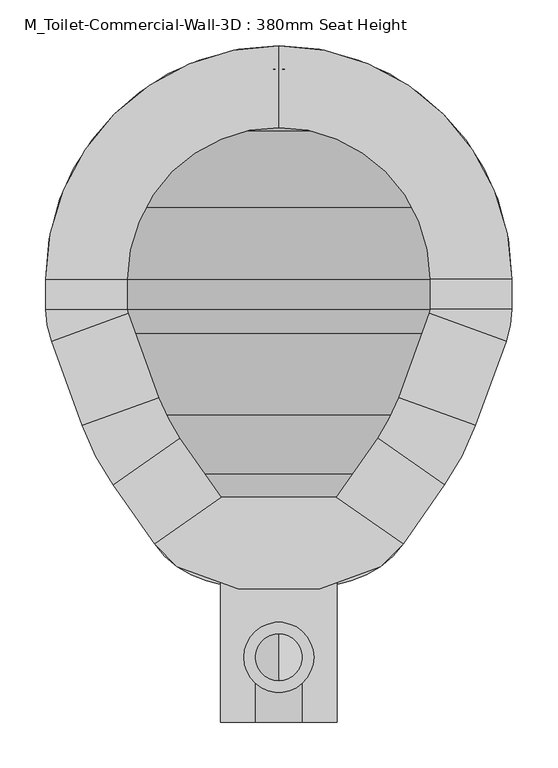
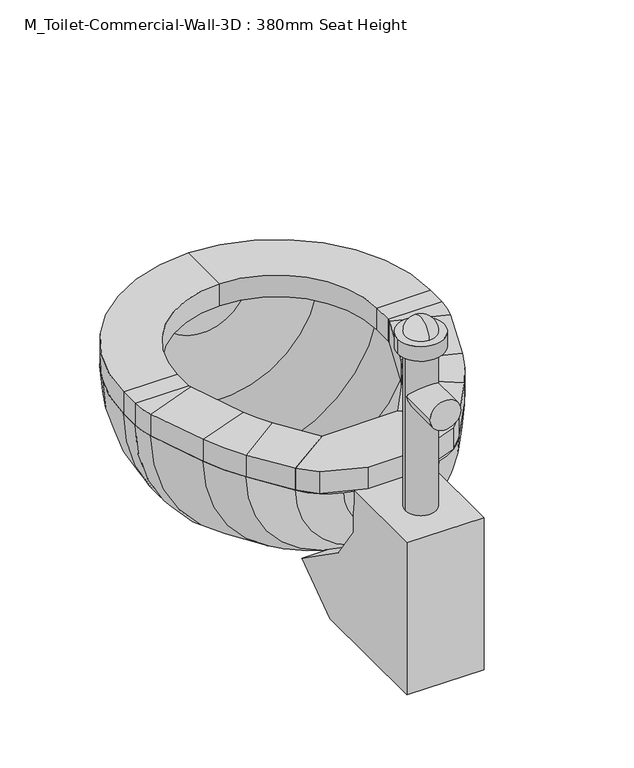
"""IFC4 building model written with IfcOpenShell, lengths in millimetres: flow terminal geometry, M_Toilet-Commercial-Wall-3D : 380mm Seat Height."""

from ifc_helpers import new_model, si_unit, point, frame, frame_2d, origin, place, context, project, spatial, polyline, circle_curve, ellipse_curve, trimmed, segment, composite_curve, outline, extrude, source, transform, mapped, element, save
from ifc_brep_helpers import plane_surface, cylinder_surface, revolved_surface, advanced_brep


def m_toilet_commercial_wall_3d_380mm_seat_height_4e8788ad(model_context):
    return source(origin(), model_context, "Body", "SolidModel", [
        extrude(outline(polyline([(302.8037941, 341.9), (302.8037941, 268.296452), (346.5103185, 205.8770663), (450.5426282, 133.0328588), (370.0454017, 76.2), (150.0, 76.2), (150.0, 341.9), (302.8037941, 341.9)])), frame((341.4031538, 0.0, 0.0), z_axis=(1.0, 0.0, 0.0), x_axis=(0.0, 1.0, 0.0)), (0.0, 0.0, 1.0), 127.0),
        extrude(outline(composite_curve([segment(trimmed(circle_curve(frame_2d((404.9031538, 220.5352737)), 25.4), [point((379.5031538, 220.5352737))], [point((430.3031538, 220.5352737))], False, "CARTESIAN"), True, "CONTINUOUS"), segment(trimmed(circle_curve(frame_2d((404.9031538, 220.5352737)), 25.4), [point((430.3031538, 220.5352737))], [point((379.5031538, 220.5352737))], False, "CARTESIAN"), True, "CONTINUOUS")], self_intersect=False)), frame((0.0, 0.0, 341.9), z_axis=(0.0, 0.0, 1.0), x_axis=(1.0, 0.0, 0.0)), (0.0, 0.0, 1.0), 279.4),
        extrude(outline(composite_curve([segment(trimmed(circle_curve(frame_2d((543.2113641, 404.9031538)), 25.4), [point((543.2113641, 379.5031538))], [point((543.2113641, 430.3031538))], False, "CARTESIAN"), True, "CONTINUOUS"), segment(trimmed(circle_curve(frame_2d((543.2113641, 404.9031538)), 25.4), [point((543.2113641, 430.3031538))], [point((543.2113641, 379.5031538))], False, "CARTESIAN"), True, "CONTINUOUS")], self_intersect=False)), frame((0.0, 150.0, 0.0), z_axis=(0.0, 1.0, 0.0), x_axis=(0.0, 0.0, 1.0)), (0.0, 0.0, 1.0), 70.64375),
        extrude(outline(composite_curve([segment(trimmed(circle_curve(frame_2d((404.9031538, 220.5352737)), 38.1), [point((366.8031538, 220.5352737))], [point((443.0031538, 220.5352737))], False, "CARTESIAN"), True, "CONTINUOUS"), segment(trimmed(circle_curve(frame_2d((404.9031538, 220.5352737)), 38.1), [point((443.0031538, 220.5352737))], [point((366.8031538, 220.5352737))], False, "CARTESIAN"), True, "CONTINUOUS")], self_intersect=False)), frame((0.0, 0.0, 621.3), z_axis=(0.0, 0.0, 1.0), x_axis=(1.0, 0.0, 0.0)), (0.0, 0.0, 1.0), 25.4),
        advanced_brep(
        [(404.9031538, 194.9176912, 646.7), (404.9031538, 246.1528563, 646.7), (404.9031538, 220.5352737, 672.3175826), (404.9031538, 220.5352737, 646.7)],
        [
            (0, 1, circle_curve(frame((404.9031538, 220.5352737, 646.7), z_axis=(0.0, 0.0, 1.0), x_axis=(0.0, 1.0, 0.0)), 25.6175826)),
            (1, 2, circle_curve(frame((404.9031538, 220.5352737, 646.7), z_axis=(1.0, 0.0, 0.0), x_axis=(0.0, -1.0, 0.0)), 25.6175826)),
            (2, 0, circle_curve(frame((404.9031538, 220.5352737, 646.7), z_axis=(1.0, 0.0, 0.0), x_axis=(0.0, 1.0, 0.0)), 25.6175826)),
            (1, 0, circle_curve(frame((404.9031538, 220.5352737, 646.7), z_axis=(0.0, 0.0, 1.0), x_axis=(0.0, 1.0, 0.0)), 25.6175826)),
            (3, 1),
            (0, 3),
        ],
        [
            revolved_surface(trimmed(ellipse_curve(frame((404.9031538, 220.5352737, 646.7), z_axis=(-1.0, 0.0, 0.0), x_axis=(0.0, -1.0, 0.0)), 25.6175826, 25.6175826), [point((404.9031538, 220.5352737, 672.3175826))], [point((404.9031538, 246.1528563, 646.7))], True, "CARTESIAN"), (404.9031538, 220.5352737, 711.3277273), (0.0, 0.0, -1.0)),
            plane_surface(frame((404.9031538, 220.5352737, 646.7), z_axis=(0.0, 0.0, -1.0), x_axis=(0.0, 1.0, 0.0))),
        ],
        [
            (0, [[1, 2, 3]]),
            (0, [[4, -3, -2]]),
            (1, [[5, -1, 6]]),
            (1, [[-6, -4, -5]]),
        ],
    ),
        advanced_brep(
        [(491.7762702, 871.2819257, 341.9), (404.9031538, 886.6, 341.9), (404.9031538, 861.2, 341.9), (483.0889586, 847.4137331, 341.9), (566.547764, 794.2446102, 341.9), (619.7168869, 710.7858048, 341.9), (633.5031538, 632.6, 341.9), (633.5031538, 599.7148212, 341.9), (628.9077315, 573.6528863, 341.9), (596.6355667, 484.9858422, 341.9), (562.9565296, 420.2890139, 341.9), (525.0728964, 366.1855786, 341.9), (468.1430637, 326.3228806, 341.9), (404.9031538, 309.3777978, 341.9), (404.9031538, 283.0817829, 341.9), (483.6469009, 304.1811063, 341.9), (540.5767337, 344.0438043, 341.9), (585.6810159, 408.4593951, 341.9), (619.360053, 473.1562234, 341.9), (652.7759241, 564.9655747, 341.9), (658.9031538, 599.7148212, 341.9), (658.9031538, 632.6, 341.9), (643.5850795, 719.4731164, 341.9), (584.5082762, 812.2051224, 341.9), (318.0300374, 871.2819257, 341.9), (225.2980314, 812.2051224, 341.9), (166.2212281, 719.4731164, 341.9), (150.9031538, 632.6, 341.9), (150.9031538, 599.7148212, 341.9), (157.0303835, 564.9655747, 341.9), (190.4462546, 473.1562234, 341.9), (224.1252917, 408.4593951, 341.9), (269.229574, 344.0438043, 341.9), (326.1594067, 304.1811063, 341.9), (341.663244, 326.3228806, 341.9), (284.7334112, 366.1855786, 341.9), (246.849778, 420.2890139, 341.9), (213.1707409, 484.9858422, 341.9), (180.8985761, 573.6528863, 341.9), (176.3031538, 599.7148212, 341.9), (176.3031538, 632.6, 341.9), (190.0894207, 710.7858048, 341.9), (243.2585436, 794.2446102, 341.9), (326.7173491, 847.4137331, 341.9)],
        [
            (0, 1, circle_curve(frame((404.9031538, 632.6, 341.9), z_axis=(0.0, 0.0, 1.0), x_axis=(1.0, 0.0, 0.0)), 254.0)),
            (1, 2),
            (2, 3, circle_curve(frame((404.9031538, 632.6, 341.9), z_axis=(0.0, 0.0, -1.0), x_axis=(1.0, 0.0, 0.0)), 228.6)),
            (3, 4, circle_curve(frame((404.9031538, 632.6, 341.9), z_axis=(0.0, 0.0, -1.0), x_axis=(1.0, 0.0, 0.0)), 228.6)),
            (4, 5, circle_curve(frame((404.9031538, 632.6, 341.9), z_axis=(0.0, 0.0, -1.0), x_axis=(1.0, 0.0, 0.0)), 228.6)),
            (5, 6, circle_curve(frame((404.9031538, 632.6, 341.9), z_axis=(0.0, 0.0, -1.0), x_axis=(1.0, 0.0, 0.0)), 228.6)),
            (6, 7),
            (7, 8, circle_curve(frame((557.3031538, 599.7148212, 341.9), z_axis=(0.0, 0.0, -1.0), x_axis=(1.0, 0.0, 0.0)), 76.2)),
            (8, 9),
            (9, 10, circle_curve(frame((334.0854485, 580.5462703, 341.9), z_axis=(0.0, 0.0, -1.0), x_axis=(1.0, 0.0, 0.0)), 279.4)),
            (10, 11),
            (11, 12, circle_curve(frame((441.8470487, 424.4609446, 341.9), z_axis=(0.0, 0.0, -1.0), x_axis=(1.0, 0.0, 0.0)), 101.6)),
            (12, 13),
            (13, 14),
            (14, 15),
            (15, 16, circle_curve(frame((457.350886, 402.3191703, 341.9), z_axis=(0.0, 0.0, 1.0), x_axis=(1.0, 0.0, 0.0)), 101.6)),
            (16, 17),
            (17, 18, circle_curve(frame((356.8099347, 568.7166514, 341.9), z_axis=(0.0, 0.0, 1.0), x_axis=(1.0, 0.0, 0.0)), 279.4)),
            (18, 19),
            (19, 20, circle_curve(frame((557.3031538, 599.7148212, 341.9), z_axis=(0.0, 0.0, 1.0), x_axis=(1.0, 0.0, 0.0)), 101.6)),
            (20, 21),
            (21, 22, circle_curve(frame((404.9031538, 632.6, 341.9), z_axis=(0.0, 0.0, 1.0), x_axis=(1.0, 0.0, 0.0)), 254.0)),
            (22, 23, circle_curve(frame((404.9031538, 632.6, 341.9), z_axis=(0.0, 0.0, 1.0), x_axis=(1.0, 0.0, 0.0)), 254.0)),
            (23, 0, circle_curve(frame((404.9031538, 632.6, 341.9), z_axis=(0.0, 0.0, 1.0), x_axis=(1.0, 0.0, 0.0)), 254.0)),
            (24, 25, circle_curve(frame((404.9031538, 632.6, 341.9), z_axis=(0.0, 0.0, 1.0), x_axis=(-1.0, 0.0, 0.0)), 254.0)),
            (25, 26, circle_curve(frame((404.9031538, 632.6, 341.9), z_axis=(0.0, 0.0, 1.0), x_axis=(-1.0, 0.0, 0.0)), 254.0)),
            (26, 27, circle_curve(frame((404.9031538, 632.6, 341.9), z_axis=(0.0, 0.0, 1.0), x_axis=(-1.0, 0.0, 0.0)), 254.0)),
            (27, 28),
            (28, 29, circle_curve(frame((252.5031538, 599.7148212, 341.9), z_axis=(0.0, 0.0, 1.0), x_axis=(-1.0, 0.0, 0.0)), 101.6)),
            (29, 30),
            (30, 31, circle_curve(frame((452.9963729, 568.7166514, 341.9), z_axis=(0.0, 0.0, 1.0), x_axis=(-1.0, 0.0, 0.0)), 279.4)),
            (31, 32),
            (32, 33, circle_curve(frame((352.4554217, 402.3191703, 341.9), z_axis=(0.0, 0.0, 1.0), x_axis=(-1.0, 0.0, 0.0)), 101.6)),
            (33, 14),
            (13, 34),
            (34, 35, circle_curve(frame((367.9592589, 424.4609446, 341.9), z_axis=(0.0, 0.0, -1.0), x_axis=(-1.0, 0.0, 0.0)), 101.6)),
            (35, 36),
            (36, 37, circle_curve(frame((475.7208592, 580.5462703, 341.9), z_axis=(0.0, 0.0, -1.0), x_axis=(-1.0, 0.0, 0.0)), 279.4)),
            (37, 38),
            (38, 39, circle_curve(frame((252.5031538, 599.7148212, 341.9), z_axis=(0.0, 0.0, -1.0), x_axis=(-1.0, 0.0, 0.0)), 76.2)),
            (39, 40),
            (40, 41, circle_curve(frame((404.9031538, 632.6, 341.9), z_axis=(0.0, 0.0, -1.0), x_axis=(-1.0, 0.0, 0.0)), 228.6)),
            (41, 42, circle_curve(frame((404.9031538, 632.6, 341.9), z_axis=(0.0, 0.0, -1.0), x_axis=(-1.0, 0.0, 0.0)), 228.6)),
            (42, 43, circle_curve(frame((404.9031538, 632.6, 341.9), z_axis=(0.0, 0.0, -1.0), x_axis=(-1.0, 0.0, 0.0)), 228.6)),
            (43, 2, circle_curve(frame((404.9031538, 632.6, 341.9), z_axis=(0.0, 0.0, -1.0), x_axis=(-1.0, 0.0, 0.0)), 228.6)),
            (1, 24, circle_curve(frame((404.9031538, 632.6, 341.9), z_axis=(0.0, 0.0, 1.0), x_axis=(-1.0, 0.0, 0.0)), 254.0)),
            (0, 24, circle_curve(frame((404.9031538, 871.2819257, 341.9), z_axis=(0.0, 1.0, 0.0), x_axis=(1.0, 0.0, 0.0)), 86.8731164)),
            (43, 3, circle_curve(frame((404.9031538, 847.4137331, 341.9), z_axis=(0.0, -1.0, 0.0), x_axis=(1.0, 0.0, 0.0)), 78.1858048)),
            (42, 4, circle_curve(frame((404.9031538, 794.2446102, 341.9), z_axis=(0.0, -1.0, 0.0), x_axis=(1.0, 0.0, 0.0)), 161.6446102)),
            (41, 5, circle_curve(frame((404.9031538, 710.7858048, 341.9), z_axis=(0.0, -1.0, 0.0), x_axis=(1.0, 0.0, 0.0)), 214.8137331)),
            (40, 6, circle_curve(frame((404.9031538, 632.6, 341.9), z_axis=(0.0, -1.0, 0.0), x_axis=(1.0, 0.0, 0.0)), 228.6)),
            (39, 7, circle_curve(frame((404.9031538, 599.7148212, 341.9), z_axis=(0.0, -1.0, 0.0), x_axis=(1.0, 0.0, 0.0)), 228.6)),
            (38, 8, circle_curve(frame((404.9031538, 573.6528863, 341.9), z_axis=(0.0, -1.0, 0.0), x_axis=(1.0, 0.0, 0.0)), 224.0045777)),
            (37, 9, circle_curve(frame((404.9031538, 484.9858422, 341.9), z_axis=(0.0, -1.0, 0.0), x_axis=(1.0, 0.0, 0.0)), 191.7324129)),
            (36, 10, circle_curve(frame((404.9031538, 420.2890139, 341.9), z_axis=(0.0, -1.0, 0.0), x_axis=(1.0, 0.0, 0.0)), 158.0533758)),
            (35, 11, circle_curve(frame((404.9031538, 366.1855786, 341.9), z_axis=(0.0, -1.0, 0.0), x_axis=(1.0, 0.0, 0.0)), 120.1697426)),
            (34, 12, circle_curve(frame((404.9031538, 326.3228806, 341.9), z_axis=(0.0, -1.0, 0.0), x_axis=(1.0, 0.0, 0.0)), 63.2399099)),
            (33, 15, circle_curve(frame((404.9031538, 304.1811063, 341.9), z_axis=(0.0, -1.0, 0.0), x_axis=(1.0, 0.0, 0.0)), 78.7437471)),
            (32, 16, circle_curve(frame((404.9031538, 344.0438043, 341.9), z_axis=(0.0, -1.0, 0.0), x_axis=(1.0, 0.0, 0.0)), 135.6735798)),
            (31, 17, circle_curve(frame((404.9031538, 408.4593951, 341.9), z_axis=(0.0, -1.0, 0.0), x_axis=(1.0, 0.0, 0.0)), 180.7778621)),
            (30, 18, circle_curve(frame((404.9031538, 473.1562234, 341.9), z_axis=(0.0, -1.0, 0.0), x_axis=(1.0, 0.0, 0.0)), 214.4568992)),
            (29, 19, circle_curve(frame((404.9031538, 564.9655747, 341.9), z_axis=(0.0, -1.0, 0.0), x_axis=(1.0, 0.0, 0.0)), 247.8727703)),
            (28, 20, circle_curve(frame((404.9031538, 599.7148212, 341.9), z_axis=(0.0, -1.0, 0.0), x_axis=(1.0, 0.0, 0.0)), 254.0)),
            (27, 21, circle_curve(frame((404.9031538, 632.6, 341.9), z_axis=(0.0, -1.0, 0.0), x_axis=(1.0, 0.0, 0.0)), 254.0)),
            (26, 22, circle_curve(frame((404.9031538, 719.4731164, 341.9), z_axis=(0.0, -1.0, 0.0), x_axis=(1.0, 0.0, 0.0)), 238.6819257)),
            (25, 23, circle_curve(frame((404.9031538, 812.2051224, 341.9), z_axis=(0.0, -1.0, 0.0), x_axis=(1.0, 0.0, 0.0)), 179.6051224)),
        ],
        [
            plane_surface(frame((404.9031538, 991.8102448, 341.9), z_axis=(0.0, 0.0, 1.0), x_axis=(1.0, 0.0, 0.0))),
            plane_surface(frame((404.9031538, 991.8102448, 341.9), z_axis=(0.0, 0.0, 1.0), x_axis=(-1.0, 0.0, 0.0))),
            revolved_surface(trimmed(ellipse_curve(frame((404.9031538, 632.6, 341.9), z_axis=(0.0, 0.0, 1.0), x_axis=(1.0, 0.0, 0.0)), 254.0, 254.0), [point((491.7762702, 871.2819257, 341.9))], [point((404.9031538, 886.6, 341.9))], True, "CARTESIAN"), (404.9031538, 991.8102448, 341.9), (0.0, 1.0, 0.0)),
            revolved_surface(trimmed(ellipse_curve(frame((404.9031538, 632.6, 341.9), z_axis=(0.0, 0.0, -1.0), x_axis=(1.0, 0.0, 0.0)), 228.6, 228.6), [point((404.9031538, 861.2, 341.9))], [point((483.0889586, 847.4137331, 341.9))], True, "CARTESIAN"), (404.9031538, 991.8102448, 341.9), (0.0, 1.0, 0.0)),
            revolved_surface(trimmed(ellipse_curve(frame((404.9031538, 632.6, 341.9), z_axis=(0.0, 0.0, -1.0), x_axis=(1.0, 0.0, 0.0)), 228.6, 228.6), [point((483.0889586, 847.4137331, 341.9))], [point((566.547764, 794.2446102, 341.9))], True, "CARTESIAN"), (404.9031538, 991.8102448, 341.9), (0.0, 1.0, 0.0)),
            revolved_surface(trimmed(ellipse_curve(frame((404.9031538, 632.6, 341.9), z_axis=(0.0, 0.0, -1.0), x_axis=(1.0, 0.0, 0.0)), 228.6, 228.6), [point((566.547764, 794.2446102, 341.9))], [point((619.7168869, 710.7858048, 341.9))], True, "CARTESIAN"), (404.9031538, 991.8102448, 341.9), (0.0, 1.0, 0.0)),
            revolved_surface(trimmed(ellipse_curve(frame((404.9031538, 632.6, 341.9), z_axis=(0.0, 0.0, -1.0), x_axis=(1.0, 0.0, 0.0)), 228.6, 228.6), [point((619.7168869, 710.7858048, 341.9))], [point((633.5031538, 632.6, 341.9))], True, "CARTESIAN"), (404.9031538, 991.8102448, 341.9), (0.0, 1.0, 0.0)),
            revolved_surface(polyline([(633.5031538, 632.6, 341.9), (633.5031538, 599.7148212, 341.9)]), (404.9031538, 991.8102448, 341.9), (0.0, 1.0, 0.0)),
            revolved_surface(trimmed(ellipse_curve(frame((557.3031538, 599.7148212, 341.9), z_axis=(0.0, 0.0, -1.0), x_axis=(1.0, 0.0, 0.0)), 76.2, 76.2), [point((633.5031538, 599.7148212, 341.9))], [point((628.9077315, 573.6528863, 341.9))], True, "CARTESIAN"), (404.9031538, 991.8102448, 341.9), (0.0, 1.0, 0.0)),
            revolved_surface(polyline([(628.9077315, 573.6528863, 341.9), (596.6355667, 484.9858422, 341.9)]), (404.9031538, 991.8102448, 341.9), (0.0, 1.0, 0.0)),
            revolved_surface(trimmed(ellipse_curve(frame((334.0854485, 580.5462703, 341.9), z_axis=(0.0, 0.0, -1.0), x_axis=(1.0, 0.0, 0.0)), 279.4, 279.4), [point((596.6355667, 484.9858422, 341.9))], [point((562.9565296, 420.2890139, 341.9))], True, "CARTESIAN"), (404.9031538, 991.8102448, 341.9), (0.0, 1.0, 0.0)),
            revolved_surface(polyline([(562.9565296, 420.2890139, 341.9), (525.0728964, 366.1855786, 341.9)]), (404.9031538, 991.8102448, 341.9), (0.0, 1.0, 0.0)),
            revolved_surface(trimmed(ellipse_curve(frame((441.8470487, 424.4609446, 341.9), z_axis=(0.0, 0.0, -1.0), x_axis=(1.0, 0.0, 0.0)), 101.6, 101.6), [point((525.0728964, 366.1855786, 341.9))], [point((468.1430637, 326.3228806, 341.9))], True, "CARTESIAN"), (404.9031538, 991.8102448, 341.9), (0.0, 1.0, 0.0)),
            revolved_surface(polyline([(468.1430637, 326.3228806, 341.9), (404.9031538, 309.3777978, 341.9)]), (404.9031538, 991.8102448, 341.9), (0.0, 1.0, 0.0)),
            revolved_surface(polyline([(404.9031538, 283.0817829, 341.9), (483.6469009, 304.1811063, 341.9)]), (404.9031538, 991.8102448, 341.9), (0.0, 1.0, 0.0)),
            revolved_surface(trimmed(ellipse_curve(frame((457.350886, 402.3191703, 341.9), z_axis=(0.0, 0.0, 1.0), x_axis=(1.0, 0.0, 0.0)), 101.6, 101.6), [point((483.6469009, 304.1811063, 341.9))], [point((540.5767337, 344.0438043, 341.9))], True, "CARTESIAN"), (404.9031538, 991.8102448, 341.9), (0.0, 1.0, 0.0)),
            revolved_surface(polyline([(540.5767337, 344.0438043, 341.9), (585.6810159, 408.4593951, 341.9)]), (404.9031538, 991.8102448, 341.9), (0.0, 1.0, 0.0)),
            revolved_surface(trimmed(ellipse_curve(frame((356.8099347, 568.7166514, 341.9), z_axis=(0.0, 0.0, 1.0), x_axis=(1.0, 0.0, 0.0)), 279.4, 279.4), [point((585.6810159, 408.4593951, 341.9))], [point((619.360053, 473.1562234, 341.9))], True, "CARTESIAN"), (404.9031538, 991.8102448, 341.9), (0.0, 1.0, 0.0)),
            revolved_surface(polyline([(619.360053, 473.1562234, 341.9), (652.7759241, 564.9655747, 341.9)]), (404.9031538, 991.8102448, 341.9), (0.0, 1.0, 0.0)),
            revolved_surface(trimmed(ellipse_curve(frame((557.3031538, 599.7148212, 341.9), z_axis=(0.0, 0.0, 1.0), x_axis=(1.0, 0.0, 0.0)), 101.6, 101.6), [point((652.7759241, 564.9655747, 341.9))], [point((658.9031538, 599.7148212, 341.9))], True, "CARTESIAN"), (404.9031538, 991.8102448, 341.9), (0.0, 1.0, 0.0)),
            cylinder_surface(frame((404.9031538, 991.8102448, 341.9), z_axis=(0.0, 1.0, 0.0), x_axis=(1.0, 0.0, 0.0)), 254.0),
            revolved_surface(trimmed(ellipse_curve(frame((404.9031538, 632.6, 341.9), z_axis=(0.0, 0.0, 1.0), x_axis=(1.0, 0.0, 0.0)), 254.0, 254.0), [point((658.9031538, 632.6, 341.9))], [point((643.5850795, 719.4731164, 341.9))], True, "CARTESIAN"), (404.9031538, 991.8102448, 341.9), (0.0, 1.0, 0.0)),
            revolved_surface(trimmed(ellipse_curve(frame((404.9031538, 632.6, 341.9), z_axis=(0.0, 0.0, 1.0), x_axis=(1.0, 0.0, 0.0)), 254.0, 254.0), [point((643.5850795, 719.4731164, 341.9))], [point((584.5082762, 812.2051224, 341.9))], True, "CARTESIAN"), (404.9031538, 991.8102448, 341.9), (0.0, 1.0, 0.0)),
            revolved_surface(trimmed(ellipse_curve(frame((404.9031538, 632.6, 341.9), z_axis=(0.0, 0.0, 1.0), x_axis=(1.0, 0.0, 0.0)), 254.0, 254.0), [point((584.5082762, 812.2051224, 341.9))], [point((491.7762702, 871.2819257, 341.9))], True, "CARTESIAN"), (404.9031538, 991.8102448, 341.9), (0.0, 1.0, 0.0)),
        ],
        [
            (0, [[1, 2, 3, 4, 5, 6, 7, 8, 9, 10, 11, 12, 13, 14, 15, 16, 17, 18, 19, 20, 21, 22, 23, 24]]),
            (1, [[25, 26, 27, 28, 29, 30, 31, 32, 33, 34, -14, 35, 36, 37, 38, 39, 40, 41, 42, 43, 44, 45, -2, 46]]),
            (2, [[-1, 47, -46]]),
            (3, [[48, -3, -45]]),
            (4, [[49, -4, -48, -44]]),
            (5, [[50, -5, -49, -43]]),
            (6, [[51, -6, -50, -42]]),
            (7, [[52, -7, -51, -41]]),
            (8, [[53, -8, -52, -40]]),
            (9, [[54, -9, -53, -39]]),
            (10, [[55, -10, -54, -38]]),
            (11, [[56, -11, -55, -37]]),
            (12, [[57, -12, -56, -36]]),
            (13, [[-13, -57, -35]]),
            (14, [[58, -15, -34]]),
            (15, [[59, -16, -58, -33]]),
            (16, [[60, -17, -59, -32]]),
            (17, [[61, -18, -60, -31]]),
            (18, [[62, -19, -61, -30]]),
            (19, [[63, -20, -62, -29]]),
            (20, [[64, -21, -63, -28]]),
            (21, [[65, -22, -64, -27]]),
            (22, [[66, -23, -65, -26]]),
            (23, [[-47, -24, -66, -25]]),
        ],
    ),
        advanced_brep(
        [(467.7541169, 395.0347495, 341.9), (540.5767337, 344.0438043, 341.9), (540.5767337, 344.0438043, 380.0), (467.7541169, 395.0347495, 380.0), (512.8583992, 459.4503403, 341.9), (585.6810159, 408.4593951, 341.9), (585.6810159, 408.4593951, 380.0), (512.8583992, 459.4503403, 380.0), (619.360053, 473.1562234, 341.9), (535.821379, 503.5618141, 341.9), (619.360053, 473.1562234, 380.0), (535.821379, 503.5618141, 380.0), (569.2372501, 595.3711654, 341.9), (652.7759241, 564.9655747, 341.9), (652.7759241, 564.9655747, 380.0), (569.2372501, 595.3711654, 380.0), (658.9031538, 599.7148212, 341.9), (570.0031538, 599.7148212, 341.9), (658.9031538, 599.7148212, 380.0), (570.0031538, 599.7148212, 380.0), (570.0031538, 632.6, 341.9), (658.9031538, 632.6, 341.9), (658.9031538, 632.6, 380.0), (570.0031538, 632.6, 380.0), (404.9031538, 886.6, 341.9), (404.9031538, 797.7, 341.9), (404.9031538, 886.6, 380.0), (404.9031538, 797.7, 380.0), (150.9031538, 632.6, 341.9), (239.8031538, 632.6, 341.9), (150.9031538, 632.6, 380.0), (239.8031538, 632.6, 380.0), (239.8031538, 599.7148212, 341.9), (150.9031538, 599.7148212, 341.9), (150.9031538, 599.7148212, 380.0), (239.8031538, 599.7148212, 380.0), (157.0303835, 564.9655747, 341.9), (240.5690575, 595.3711654, 341.9), (157.0303835, 564.9655747, 380.0), (240.5690575, 595.3711654, 380.0), (273.9849286, 503.5618141, 341.9), (190.4462546, 473.1562234, 341.9), (190.4462546, 473.1562234, 380.0), (273.9849286, 503.5618141, 380.0), (224.1252917, 408.4593951, 341.9), (296.9479084, 459.4503403, 341.9), (224.1252917, 408.4593951, 380.0), (296.9479084, 459.4503403, 380.0), (342.0521907, 395.0347495, 341.9), (342.0521907, 395.0347495, 380.0), (269.229574, 344.0438043, 380.0), (269.229574, 344.0438043, 341.9)],
        [
            (0, 1),
            (1, 2),
            (2, 3),
            (3, 0),
            (0, 4),
            (4, 5),
            (5, 1),
            (5, 6),
            (6, 2),
            (6, 7),
            (7, 3),
            (7, 4),
            (8, 5, circle_curve(frame((356.8099347, 568.7166514, 341.9), z_axis=(0.0, 0.0, -1.0), x_axis=(0.819152044288991, -0.5735764363510472, 0.0)), 279.4)),
            (4, 9, circle_curve(frame((356.8099347, 568.7166514, 341.9), z_axis=(0.0, 0.0, 1.0), x_axis=(0.819152044288991, -0.5735764363510472, 0.0)), 190.5)),
            (9, 8),
            (10, 6, circle_curve(frame((356.8099347, 568.7166514, 380.0), z_axis=(0.0, 0.0, -1.0), x_axis=(0.819152044288991, -0.5735764363510472, 0.0)), 279.4)),
            (8, 10),
            (11, 7, circle_curve(frame((356.8099347, 568.7166514, 380.0), z_axis=(0.0, 0.0, -1.0), x_axis=(0.819152044288991, -0.5735764363510472, 0.0)), 190.5)),
            (10, 11),
            (11, 9),
            (9, 12),
            (12, 13),
            (13, 8),
            (13, 14),
            (14, 10),
            (14, 15),
            (15, 11),
            (15, 12),
            (16, 13, circle_curve(frame((557.3031538, 599.7148212, 341.9), z_axis=(0.0, 0.0, -1.0), x_axis=(0.93969262078591, -0.3420201433256644, 0.0)), 101.6)),
            (12, 17, circle_curve(frame((557.3031538, 599.7148212, 341.9), z_axis=(0.0, 0.0, 1.0), x_axis=(0.93969262078591, -0.3420201433256644, 0.0)), 12.7)),
            (17, 16),
            (18, 14, circle_curve(frame((557.3031538, 599.7148212, 380.0), z_axis=(0.0, 0.0, -1.0), x_axis=(0.93969262078591, -0.3420201433256644, 0.0)), 101.6)),
            (16, 18),
            (19, 15, circle_curve(frame((557.3031538, 599.7148212, 380.0), z_axis=(0.0, 0.0, -1.0), x_axis=(0.93969262078591, -0.3420201433256644, 0.0)), 12.7)),
            (18, 19),
            (19, 17),
            (17, 20),
            (20, 21),
            (21, 16),
            (21, 22),
            (22, 18),
            (22, 23),
            (23, 19),
            (23, 20),
            (24, 21, circle_curve(frame((404.9031538, 632.6, 341.9), z_axis=(0.0, 0.0, -1.0), x_axis=(1.0, 0.0, 0.0)), 254.0)),
            (20, 25, circle_curve(frame((404.9031538, 632.6, 341.9), z_axis=(0.0, 0.0, 1.0), x_axis=(1.0, 0.0, 0.0)), 165.1)),
            (25, 24),
            (26, 22, circle_curve(frame((404.9031538, 632.6, 380.0), z_axis=(0.0, 0.0, -1.0), x_axis=(1.0, 0.0, 0.0)), 254.0)),
            (24, 26),
            (27, 23, circle_curve(frame((404.9031538, 632.6, 380.0), z_axis=(0.0, 0.0, -1.0), x_axis=(1.0, 0.0, 0.0)), 165.1)),
            (26, 27),
            (27, 25),
            (28, 24, circle_curve(frame((404.9031538, 632.6, 341.9), z_axis=(0.0, 0.0, -1.0), x_axis=(0.0, 1.0, 0.0)), 254.0)),
            (25, 29, circle_curve(frame((404.9031538, 632.6, 341.9), z_axis=(0.0, 0.0, 1.0), x_axis=(0.0, 1.0, 0.0)), 165.1)),
            (29, 28),
            (30, 26, circle_curve(frame((404.9031538, 632.6, 380.0), z_axis=(0.0, 0.0, -1.0), x_axis=(0.0, 1.0, 0.0)), 254.0)),
            (28, 30),
            (31, 27, circle_curve(frame((404.9031538, 632.6, 380.0), z_axis=(0.0, 0.0, -1.0), x_axis=(0.0, 1.0, 0.0)), 165.1)),
            (30, 31),
            (31, 29),
            (29, 32),
            (32, 33),
            (33, 28),
            (33, 34),
            (34, 30),
            (34, 35),
            (35, 31),
            (35, 32),
            (36, 33, circle_curve(frame((252.5031538, 599.7148212, 341.9), z_axis=(0.0, 0.0, -1.0), x_axis=(-1.0, 0.0, 0.0)), 101.6)),
            (32, 37, circle_curve(frame((252.5031538, 599.7148212, 341.9), z_axis=(0.0, 0.0, 1.0), x_axis=(-1.0, 0.0, 0.0)), 12.7)),
            (37, 36),
            (38, 34, circle_curve(frame((252.5031538, 599.7148212, 380.0), z_axis=(0.0, 0.0, -1.0), x_axis=(-1.0, 0.0, 0.0)), 101.6)),
            (36, 38),
            (39, 35, circle_curve(frame((252.5031538, 599.7148212, 380.0), z_axis=(0.0, 0.0, -1.0), x_axis=(-1.0, 0.0, 0.0)), 12.7)),
            (38, 39),
            (39, 37),
            (37, 40),
            (40, 41),
            (41, 36),
            (41, 42),
            (42, 38),
            (42, 43),
            (43, 39),
            (43, 40),
            (44, 41, circle_curve(frame((452.9963729, 568.7166514, 341.9), z_axis=(0.0, 0.0, -1.0), x_axis=(-0.9396926207859084, -0.3420201433256685, 0.0)), 279.4)),
            (40, 45, circle_curve(frame((452.9963729, 568.7166514, 341.9), z_axis=(0.0, 0.0, 1.0), x_axis=(-0.9396926207859084, -0.3420201433256685, 0.0)), 190.5)),
            (45, 44),
            (46, 42, circle_curve(frame((452.9963729, 568.7166514, 380.0), z_axis=(0.0, 0.0, -1.0), x_axis=(-0.9396926207859084, -0.3420201433256685, 0.0)), 279.4)),
            (44, 46),
            (47, 43, circle_curve(frame((452.9963729, 568.7166514, 380.0), z_axis=(0.0, 0.0, -1.0), x_axis=(-0.9396926207859084, -0.3420201433256685, 0.0)), 190.5)),
            (46, 47),
            (47, 45),
            (48, 49),
            (49, 50),
            (50, 51),
            (51, 48),
            (45, 48),
            (51, 44),
            (50, 46),
            (49, 47),
        ],
        [
            plane_surface(frame((540.5767337, 344.0438043, 438.6203184), z_axis=(-0.5735764363510417, -0.8191520442889948, 0.0), x_axis=(0.8191520442889948, -0.5735764363510417, 0.0))),
            plane_surface(frame((467.7541169, 395.0347495, 341.9), z_axis=(0.0, 0.0, -1.0000000000000002), x_axis=(0.5735764363510419, 0.8191520442889948, 0.0))),
            plane_surface(frame((540.5767337, 344.0438043, 341.9), z_axis=(0.8191520442889948, -0.5735764363510419, 0.0), x_axis=(0.5735764363510419, 0.8191520442889948, 0.0))),
            plane_surface(frame((540.5767337, 344.0438043, 380.0), z_axis=(0.0, 0.0, 1.0000000000000002), x_axis=(0.5735764363510419, 0.8191520442889948, 0.0))),
            plane_surface(frame((467.7541169, 395.0347495, 380.0), z_axis=(-0.8191520442889946, 0.5735764363510424, 0.0), x_axis=(0.5735764363510424, 0.8191520442889946, 0.0))),
            plane_surface(frame((356.8099347, 568.7166514, 341.9), z_axis=(0.0, 0.0, -1.0), x_axis=(0.819152044288991, -0.5735764363510472, 0.0))),
            cylinder_surface(frame((356.8099347, 568.7166514, 341.9), z_axis=(0.0, 0.0, 1.0), x_axis=(0.819152044288991, -0.5735764363510472, 0.0)), 279.4),
            plane_surface(frame((356.8099347, 568.7166514, 380.0), z_axis=(0.0, 0.0, 1.0), x_axis=(0.819152044288991, -0.5735764363510472, 0.0))),
            revolved_surface(polyline([(512.8583991370527, 459.45034027512554, 380.0), (512.8583991370527, 459.45034027512554, 341.9)]), (356.8099347, 568.7166514, 341.9), (0.0, 0.0, 1.0)),
            plane_surface(frame((535.821379, 503.5618141, 341.9), z_axis=(0.0, 0.0, -1.0000000000000002), x_axis=(0.342020143325635, 0.9396926207859208, 0.0))),
            plane_surface(frame((619.360053, 473.1562234, 341.9), z_axis=(0.939692620785921, -0.342020143325634, 0.0), x_axis=(0.342020143325634, 0.939692620785921, 0.0))),
            plane_surface(frame((619.360053, 473.1562234, 380.0), z_axis=(0.0, 0.0, 1.0), x_axis=(0.342020143325634, 0.939692620785921, 0.0))),
            plane_surface(frame((535.821379, 503.5618141, 380.0), z_axis=(-0.9396926207859208, 0.3420201433256348, 0.0), x_axis=(0.3420201433256348, 0.9396926207859208, 0.0))),
            plane_surface(frame((557.3031538, 599.7148212, 341.9), z_axis=(0.0, 0.0, -1.0), x_axis=(0.93969262078591, -0.3420201433256644, 0.0))),
            cylinder_surface(frame((557.3031538, 599.7148212, 341.9), z_axis=(0.0, 0.0, 1.0), x_axis=(0.93969262078591, -0.3420201433256644, 0.0)), 101.6),
            plane_surface(frame((557.3031538, 599.7148212, 380.0), z_axis=(0.0, 0.0, 1.0), x_axis=(0.93969262078591, -0.3420201433256644, 0.0))),
            revolved_surface(polyline([(569.237250083981, 595.3711653797641, 380.0), (569.237250083981, 595.3711653797641, 341.9)]), (557.3031538, 599.7148212, 341.9), (0.0, 0.0, 1.0)),
            plane_surface(frame((570.0031538, 599.7148212, 341.9), z_axis=(0.0, 0.0, -1.0), x_axis=(0.0, 1.0, 0.0))),
            plane_surface(frame((658.9031538, 599.7148212, 341.9), z_axis=(1.0, 0.0, 0.0), x_axis=(0.0, 1.0, 0.0))),
            plane_surface(frame((658.9031538, 599.7148212, 380.0), z_axis=(0.0, 0.0, 1.0), x_axis=(0.0, 1.0, 0.0))),
            plane_surface(frame((570.0031538, 599.7148212, 380.0), z_axis=(-1.0, 0.0, 0.0), x_axis=(0.0, 1.0, 0.0))),
            plane_surface(frame((404.9031538, 632.6, 341.9), z_axis=(0.0, 0.0, -1.0), x_axis=(1.0, 0.0, 0.0))),
            cylinder_surface(frame((404.9031538, 632.6, 341.9), z_axis=(0.0, 0.0, 1.0), x_axis=(1.0, 0.0, 0.0)), 254.0),
            plane_surface(frame((404.9031538, 632.6, 380.0), z_axis=(0.0, 0.0, 1.0), x_axis=(1.0, 0.0, 0.0))),
            revolved_surface(polyline([(570.0031538, 632.6, 380.0), (570.0031538, 632.6, 341.9)]), (404.9031538, 632.6, 341.9), (0.0, 0.0, 1.0)),
            plane_surface(frame((404.9031538, 632.6, 341.9), z_axis=(0.0, 0.0, -1.0), x_axis=(0.0, 1.0, 0.0))),
            cylinder_surface(frame((404.9031538, 632.6, 341.9), z_axis=(0.0, 0.0, 1.0), x_axis=(0.0, 1.0, 0.0)), 254.0),
            plane_surface(frame((404.9031538, 632.6, 380.0), z_axis=(0.0, 0.0, 1.0), x_axis=(0.0, 1.0, 0.0))),
            revolved_surface(polyline([(404.9031538, 797.7, 380.0), (404.9031538, 797.7, 341.9)]), (404.9031538, 632.6, 341.9), (0.0, 0.0, 1.0)),
            plane_surface(frame((239.8031538, 632.6, 341.9), z_axis=(0.0, 0.0, -1.0), x_axis=(0.0, -1.0, 0.0))),
            plane_surface(frame((150.9031538, 632.6, 341.9), z_axis=(-1.0, 0.0, 0.0), x_axis=(0.0, -1.0, 0.0))),
            plane_surface(frame((150.9031538, 632.6, 380.0), z_axis=(0.0, 0.0, 1.0), x_axis=(0.0, -1.0, 0.0))),
            plane_surface(frame((239.8031538, 632.6, 380.0), z_axis=(1.0, 0.0, 0.0), x_axis=(0.0, -1.0, 0.0))),
            plane_surface(frame((252.5031538, 599.7148212, 341.9), z_axis=(0.0, 0.0, -1.0), x_axis=(-1.0, 0.0, 0.0))),
            cylinder_surface(frame((252.5031538, 599.7148212, 341.9), z_axis=(0.0, 0.0, 1.0), x_axis=(-1.0, 0.0, 0.0)), 101.6),
            plane_surface(frame((252.5031538, 599.7148212, 380.0), z_axis=(0.0, 0.0, 1.0), x_axis=(-1.0, 0.0, 0.0))),
            revolved_surface(polyline([(239.80315380000002, 599.7148212, 380.0), (239.80315380000002, 599.7148212, 341.9)]), (252.5031538, 599.7148212, 341.9), (0.0, 0.0, 1.0)),
            plane_surface(frame((240.5690575, 595.3711654, 341.9), z_axis=(0.0, 0.0, -1.0), x_axis=(0.3420201433256614, -0.9396926207859111, 0.0))),
            plane_surface(frame((157.0303835, 564.9655747, 341.9), z_axis=(-0.9396926207859111, -0.3420201433256614, 0.0), x_axis=(0.3420201433256614, -0.9396926207859111, 0.0))),
            plane_surface(frame((157.0303835, 564.9655747, 380.0), z_axis=(0.0, 0.0, 1.0), x_axis=(0.3420201433256611, -0.9396926207859112, 0.0))),
            plane_surface(frame((240.5690575, 595.3711654, 380.0), z_axis=(0.9396926207859112, 0.34202014332566105, 0.0), x_axis=(0.34202014332566105, -0.9396926207859112, 0.0))),
            plane_surface(frame((452.9963729, 568.7166514, 341.9), z_axis=(0.0, 0.0, -1.0000000000000002), x_axis=(-0.9396926207859085, -0.34202014332566855, 0.0))),
            cylinder_surface(frame((452.9963729, 568.7166514, 341.9), z_axis=(0.0, 0.0, 1.0), x_axis=(-0.9396926207859084, -0.3420201433256685, 0.0)), 279.4),
            plane_surface(frame((452.9963729, 568.7166514, 380.0), z_axis=(0.0, 0.0, 1.0000000000000002), x_axis=(-0.9396926207859085, -0.34202014332566855, 0.0))),
            revolved_surface(polyline([(273.98492864028447, 503.5618140964602, 380.0), (273.98492864028447, 503.5618140964602, 341.9)]), (452.9963729, 568.7166514, 341.9), (0.0, 0.0, 1.0)),
            plane_surface(frame((269.229574, 344.0438043, 245.1796816), z_axis=(0.5735764363510485, -0.8191520442889902, 0.0), x_axis=(0.8191520442889902, 0.5735764363510485, 0.0))),
            plane_surface(frame((296.9479084, 459.4503403, 341.9), z_axis=(0.0, 0.0, -1.0), x_axis=(0.5735764363510486, -0.81915204428899, 0.0))),
            plane_surface(frame((224.1252917, 408.4593951, 341.9), z_axis=(-0.8191520442889904, -0.5735764363510483, 0.0), x_axis=(0.5735764363510483, -0.8191520442889904, 0.0))),
            plane_surface(frame((224.1252917, 408.4593951, 380.0), z_axis=(0.0, 0.0, 1.0), x_axis=(0.5735764363510492, -0.8191520442889897, 0.0))),
            plane_surface(frame((296.9479084, 459.4503403, 380.0), z_axis=(0.81915204428899, 0.5735764363510486, 0.0), x_axis=(0.5735764363510486, -0.81915204428899, 0.0))),
        ],
        [
            (0, [[1, 2, 3, 4]]),
            (1, [[-1, 5, 6, 7]]),
            (2, [[-2, -7, 8, 9]]),
            (3, [[-3, -9, 10, 11]]),
            (4, [[-4, -11, 12, -5]]),
            (5, [[13, -6, 14, 15]]),
            (6, [[16, -8, -13, 17]]),
            (7, [[18, -10, -16, 19]]),
            (8, [[-14, -12, -18, 20]]),
            (9, [[-15, 21, 22, 23]]),
            (10, [[-17, -23, 24, 25]]),
            (11, [[-19, -25, 26, 27]]),
            (12, [[-20, -27, 28, -21]]),
            (13, [[29, -22, 30, 31]]),
            (14, [[32, -24, -29, 33]]),
            (15, [[34, -26, -32, 35]]),
            (16, [[-30, -28, -34, 36]]),
            (17, [[-31, 37, 38, 39]]),
            (18, [[-33, -39, 40, 41]]),
            (19, [[-35, -41, 42, 43]]),
            (20, [[-36, -43, 44, -37]]),
            (21, [[45, -38, 46, 47]]),
            (22, [[48, -40, -45, 49]]),
            (23, [[50, -42, -48, 51]]),
            (24, [[-46, -44, -50, 52]]),
            (25, [[53, -47, 54, 55]]),
            (26, [[56, -49, -53, 57]]),
            (27, [[58, -51, -56, 59]]),
            (28, [[-54, -52, -58, 60]]),
            (29, [[-55, 61, 62, 63]]),
            (30, [[-57, -63, 64, 65]]),
            (31, [[-59, -65, 66, 67]]),
            (32, [[-60, -67, 68, -61]]),
            (33, [[69, -62, 70, 71]]),
            (34, [[72, -64, -69, 73]]),
            (35, [[74, -66, -72, 75]]),
            (36, [[-70, -68, -74, 76]]),
            (37, [[-71, 77, 78, 79]]),
            (38, [[-73, -79, 80, 81]]),
            (39, [[-75, -81, 82, 83]]),
            (40, [[-76, -83, 84, -77]]),
            (41, [[85, -78, 86, 87]]),
            (42, [[88, -80, -85, 89]]),
            (43, [[90, -82, -88, 91]]),
            (44, [[-86, -84, -90, 92]]),
            (45, [[93, 94, 95, 96]]),
            (46, [[-87, 97, -96, 98]]),
            (47, [[-89, -98, -95, 99]]),
            (48, [[-91, -99, -94, 100]]),
            (49, [[-92, -100, -93, -97]]),
        ],
    ),
        extrude(outline(polyline([(467.7541169, 395.0347495), (540.5767337, 344.0438043), (515.6262519, 319.0933226), (449.563909, 295.0485961), (360.2423986, 295.0485961), (294.1800557, 319.0933226), (269.229574, 344.0438043), (342.0521907, 395.0347495), (467.7541169, 395.0347495)])), frame((0.0, 0.0, 341.9), z_axis=(0.0, 0.0, 1.0), x_axis=(1.0, 0.0, 0.0)), (0.0, 0.0, 1.0), 38.1),
    ])


if __name__ == "__main__":
    model = new_model("IFC4")
    model_context = context("Model", 3, world=origin())
    ifc_project = project(units=[si_unit("LENGTHUNIT", "METRE", prefix="MILLI")], contexts=[model_context])
    site = spatial("IfcSite", under=ifc_project)
    building = spatial("IfcBuilding", under=site)
    placement = place(None, origin())
    m_toilet_commercial_wall_3d_380mm_seat_height_shape = m_toilet_commercial_wall_3d_380mm_seat_height_4e8788ad(model_context)
    element("IfcFlowTerminal", 1, ObjectType="M_Toilet-Commercial-Wall-3D : 380mm Seat Height", at=placement, inside=building, context=model_context, shape_type="MappedRepresentation", body=[
        mapped(m_toilet_commercial_wall_3d_380mm_seat_height_shape, transform((0.0, 0.0, 0.0), x_axis=(1.0, 0.0, 0.0), y_axis=(0.0, 1.0, 0.0), z_axis=(0.0, 0.0, 1.0))),
    ])
    save(model, "model.ifc")

# Revit data of these elements
# Type "M_Toilet-Commercial-Wall-3D : 380mm Seat Height"
#   Mounting Height = 380 mm
#   Piping Material = Steel, Polished
#   Bowl Material = Porcelain, Ivory
#   Seat Material = Laminate, Ivory, Matte
#   Default Elevation = 0
# Element 1 (IfcFlowTerminal, "M_Toilet-Commercial-Wall-3D : 380mm Seat Height")
#   Materials on its faces: "Laminate, Ivory, Matte", "Porcelain, Ivory", "Steel, Polished"
# Materials
#   "Steel, Polished": class "Metal", colour RGB 57 57 57, transparency 0, Description = "Polished steel", Cost = 0
#   "Porcelain, Ivory": class "Ceramic", colour RGB 247 247 239, transparency 0, Description = "Porcelain, ivory", Cost = 0
#   "Laminate, Ivory, Matte": class "Plastic", colour RGB 247 247 239, transparency 0, Description = "Plastic Laminate - Ivory, Matte", Cost = 0
